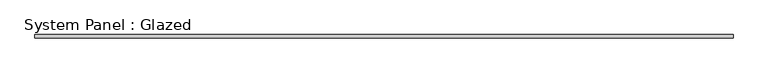
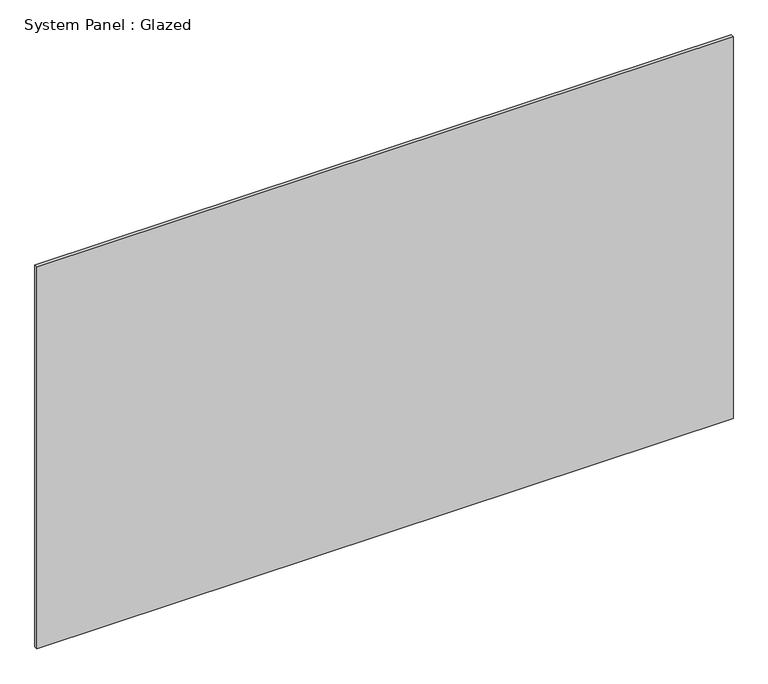
"""IFC4 building model written with IfcOpenShell, lengths in millimetres: plate geometry, System Panel : Glazed."""

from ifc_helpers import new_model, si_unit, origin, origin_with_axes, place, context, project, spatial, polyline, outline, extrude, source, transform, mapped, element, save


def system_panel_glazed_2002d5d4(model_context):
    return source(origin(), model_context, "Body", "SweptSolid", [
        extrude(outline(polyline([(2628.9, 19.05), (-2628.9, 19.05), (-2628.9, 44.45), (2628.9, 44.45), (2628.9, 19.05)])), origin_with_axes(), (0.0, 0.0, 1.0), 3048.0),
    ])


if __name__ == "__main__":
    model = new_model("IFC4")
    model_context = context("Model", 3, world=origin())
    ifc_project = project(units=[si_unit("LENGTHUNIT", "METRE", prefix="MILLI")], contexts=[model_context])
    site = spatial("IfcSite", under=ifc_project)
    building = spatial("IfcBuilding", under=site)
    placement = place(None, origin())
    system_panel_glazed_shape = system_panel_glazed_2002d5d4(model_context)
    element("IfcPlate", 1, ObjectType="System Panel : Glazed", at=placement, inside=building, context=model_context, shape_type="MappedRepresentation", body=[
        mapped(system_panel_glazed_shape, transform((0.0, 0.0, 0.0), x_axis=(1.0, 0.0, 0.0), y_axis=(0.0, 1.0, 0.0), z_axis=(0.0, 0.0, 1.0))),
    ])
    save(model, "model.ifc")

# Revit data of these elements
# Type "System Panel : Glazed"
#   Construction Type Id = "GSP4R"
#   Analytic Construction = "1/8 in Pilkington single glazing"
#   Visual Light Transmittance = 0.9
#   Solar Heat Gain Coefficient = 0.86
#   Heat Transfer Coefficient (U) = 1.18115 BTU/(h·ft²·°F)
# Element 1 (IfcPlate, "System Panel : Glazed")
#   Materials on its faces: "Glass"
# Materials
#   "Glass": class "Glass", colour RGB 0 128 192, transparency 0.75, Description = "Soda Lime Glass", Cost = 0
